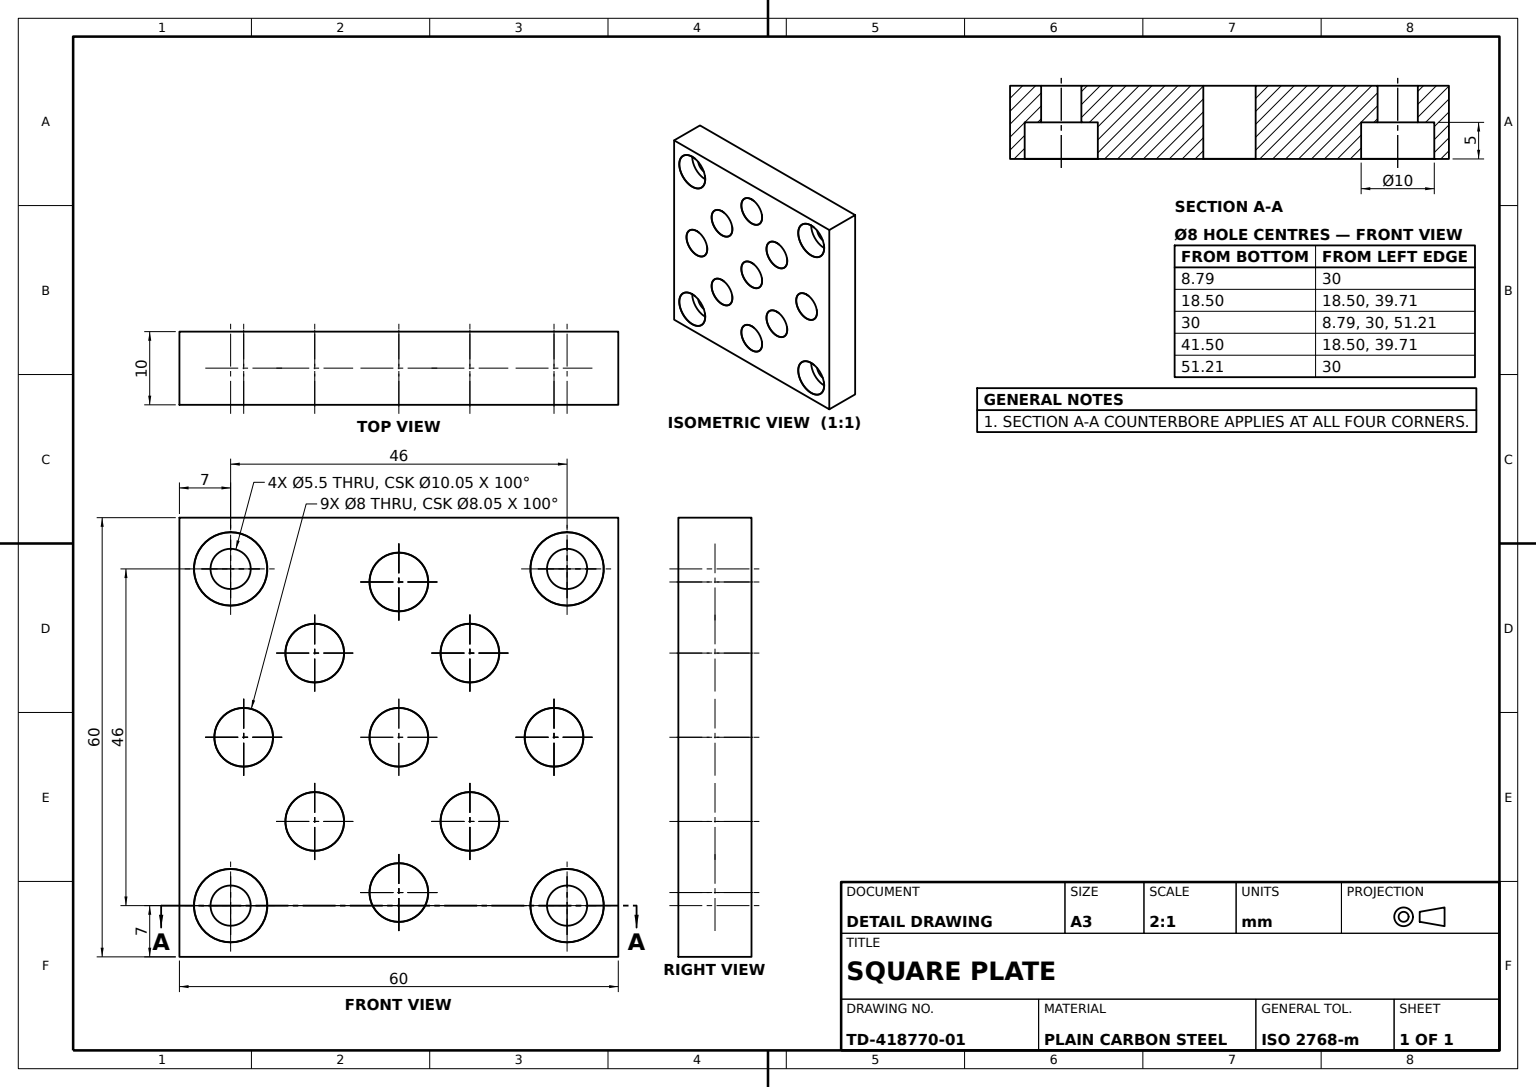
from build123d import *

# Parameters (mm, degrees)
BASE_PLATE_PROFILE_W                   = 60
BASE_PLATE_PROFILE_H                   = 60
BASE_PLATE_60X60X10_DEPTH              = 10
CORNER_COUNTERBORES_M5_SHCS_AT_2_COUNT = 2
CORNER_COUNTERBORES_M5_SHCS_AT_2_PITCH = 46
CORNER_COUNTERBORES_M5_SHCS_AT_3_COUNT = 2
CORNER_COUNTERBORES_M5_SHCS_AT_3_PITCH = 65.053823869
CORNER_COUNTERBORES_M5_SHCS_AT_4_COUNT = 2
CORNER_COUNTERBORES_M5_SHCS_AT_4_PITCH = 46
DOWEL_HOLE_GRID_8_D                    = 8
DOWEL_HOLE_GRID_8_DEPTH                = 35.596557524
DOWEL_HOLE_GRID_8_CSINK_D              = 8.05
DOWEL_HOLE_GRID_8_CSINK_ANGLE          = 100
DOWEL_HOLE_GRID_8_TIP                  = 2.403442476


with BuildPart() as part:
    # Base Plate Profile → Base Plate 60x60x10 (new body)
    with BuildSketch(Plane(origin=(0, 0, 0), x_dir=(1, 0, 0), z_dir=(0, 1, 0))):
        Rectangle(BASE_PLATE_PROFILE_W, BASE_PLATE_PROFILE_H)
    extrude(amount=BASE_PLATE_60X60X10_DEPTH)

    # Sketch3 → Corner Counterbores M5 SHCS (revolve, cut)
    with BuildSketch(Plane(origin=(-23, 10, -23), x_dir=(0, 0, 1), z_dir=(1, 0, 0))):
        Polygon((0, 0), (0, 38), (2.75, 36.347633298), (2.75, 5), (5, 5), (5, 0.020977491), (5.025, 0), align=None)
    corner_counterbores_m5_shcs = revolve(axis=Axis((-23, 16.35, -23), (0, -1, 0)), mode=Mode.SUBTRACT)

    # Corner Counterbores M5 SHCS at 2: Corner Counterbores M5 SHCS ×2
    with Locations(*[(i * CORNER_COUNTERBORES_M5_SHCS_AT_2_PITCH, 0, 0) for i in range(1, CORNER_COUNTERBORES_M5_SHCS_AT_2_COUNT)]):
        add(corner_counterbores_m5_shcs, mode=Mode.SUBTRACT)

    # Corner Counterbores M5 SHCS at 3: Corner Counterbores M5 SHCS ×2
    with Locations(*[Vector(0.7071067811865476, 0, 0.7071067811865476) * (i * CORNER_COUNTERBORES_M5_SHCS_AT_3_PITCH) for i in range(1, CORNER_COUNTERBORES_M5_SHCS_AT_3_COUNT)]):
        add(corner_counterbores_m5_shcs, mode=Mode.SUBTRACT)

    # Corner Counterbores M5 SHCS at 4: Corner Counterbores M5 SHCS ×2
    with Locations(*[(0, 0, i * CORNER_COUNTERBORES_M5_SHCS_AT_4_PITCH) for i in range(1, CORNER_COUNTERBORES_M5_SHCS_AT_4_COUNT)]):
        add(corner_counterbores_m5_shcs, mode=Mode.SUBTRACT)

    # Dowel Hole Grid Ø8
    with Locations(Plane(origin=(0, 10, 0), x_dir=(1, 0, 0), z_dir=(0, 1, 0))):
        with Locations((-21.213203436, 0), (0, 0), (21.213203436, 0), (-11.5, 11.5), (9.713203436, 11.5), (0, 21.213203436), (-11.5, -11.5), (9.713203436, -11.5), (0, -21.213203436)):
            CounterSinkHole(DOWEL_HOLE_GRID_8_D / 2, DOWEL_HOLE_GRID_8_CSINK_D / 2, depth=DOWEL_HOLE_GRID_8_DEPTH, counter_sink_angle=DOWEL_HOLE_GRID_8_CSINK_ANGLE)
            with Locations((0, 0, -(DOWEL_HOLE_GRID_8_DEPTH + DOWEL_HOLE_GRID_8_TIP / 2))):  # 118° drill point
                Cone(0, DOWEL_HOLE_GRID_8_D / 2, DOWEL_HOLE_GRID_8_TIP, mode=Mode.SUBTRACT)


solid = part.part
